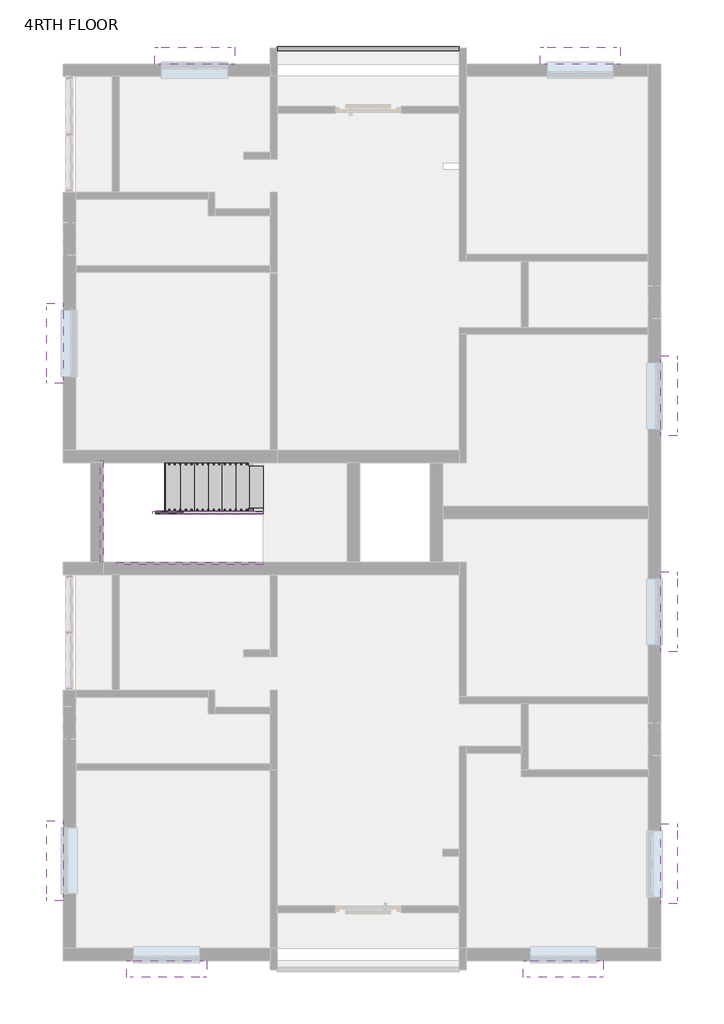
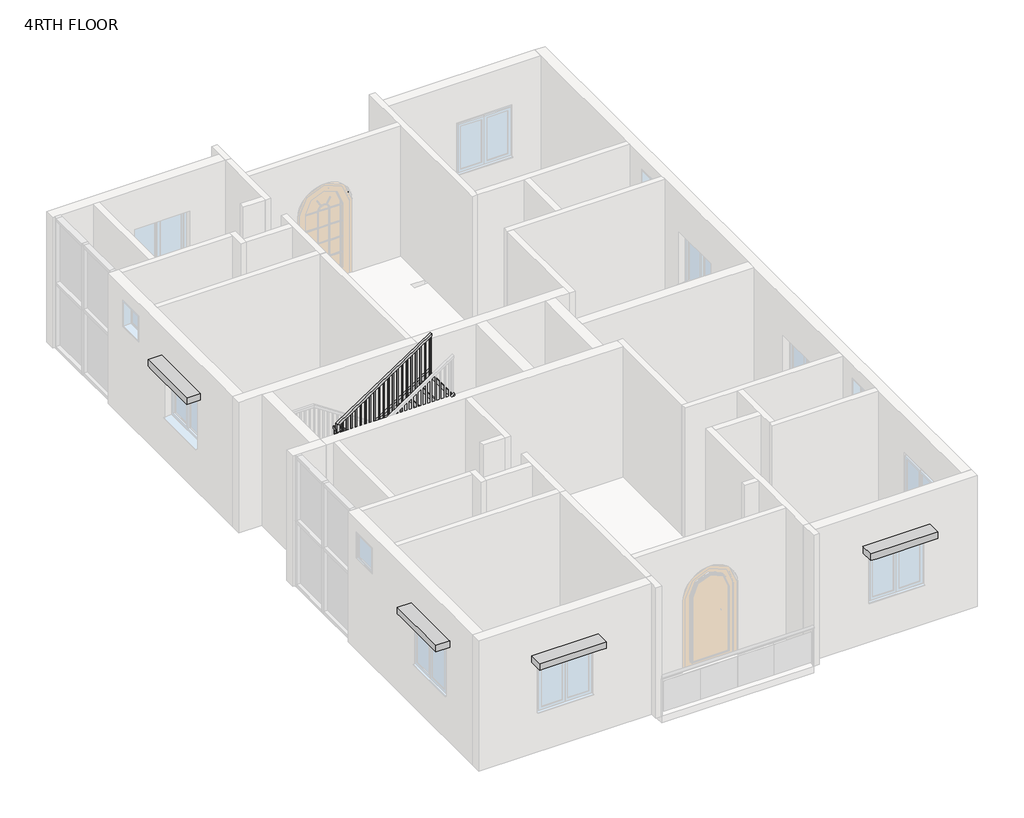
# One storey, part 4 of 4: 9 proxies, 5 members, 2 railings, 1 stair flight.
"""IFC4 building model written with IfcOpenShell, lengths in millimetres."""

from ifc_helpers import new_model, si_unit, point, frame, origin, place, context, project, spatial, polyline, ellipse_curve, trimmed, outline, extrude, faceted_brep, transform, mapped, element, save
from ifc_brep_helpers import plane_surface, extruded_surface, advanced_brep
from components import generic_models_1_generic_models_1_fbb7ad13, generic_models_11_generic_models_11_d301a5e8, generic_models_21_generic_models_21_87948dc1, generic_models_36_generic_models_36_9c63594f, stair_flight_f55dda53

model = new_model("IFC4")

# Units and contexts
model_context = context("Model", 3, world=origin())
ifc_project = project(units=[si_unit("LENGTHUNIT", "METRE", prefix="MILLI")], contexts=[model_context])

# Site, building, storey
site = spatial("IfcSite", under=ifc_project)
building = spatial("IfcBuilding", under=site)
storey = spatial("IfcBuildingStorey", under=building, Name="4RTH FLOOR", Elevation=15240.0)

# Proxies
placement = place(None, origin())
generic_models_1_generic_models_1_shape = generic_models_1_generic_models_1_fbb7ad13(model_context)
element("IfcBuildingElementProxy", 1, Name="Generic Models 1 : Generic Models 1", ObjectType="Generic Models 1 : Generic Models 1", at=placement, inside=storey, context=model_context, shape_type="MappedRepresentation", body=[
    mapped(generic_models_1_generic_models_1_shape, transform((0.0, 0.0, 0.0), x_axis=(1.0, 0.0, 0.0), y_axis=(0.0, 1.0, 0.0), z_axis=(0.0, 0.0, 1.0))),
])
generic_models_11_generic_models_11_shape = generic_models_11_generic_models_11_d301a5e8(model_context)
element("IfcBuildingElementProxy", 2, Name="Generic Models 11 : Generic Models 11", ObjectType="Generic Models 11 : Generic Models 11", at=placement, inside=storey, context=model_context, shape_type="MappedRepresentation", body=[
    mapped(generic_models_11_generic_models_11_shape, transform((0.0, 0.0, 0.0), x_axis=(1.0, 0.0, 0.0), y_axis=(0.0, 1.0, 0.0), z_axis=(0.0, 0.0, 1.0))),
])
element("IfcBuildingElementProxy", 3, Name="Generic Models 12 : Generic Models 11", ObjectType="Generic Models 12 : Generic Models 11", at=placement, inside=storey, context=model_context, shape_type="MappedRepresentation", body=[
    mapped(generic_models_11_generic_models_11_shape, transform((-7101.0359618, 0.0, 0.0), x_axis=(1.0, 0.0, 0.0), y_axis=(0.0, 1.0, 0.0), z_axis=(0.0, 0.0, 1.0))),
])
element("IfcBuildingElementProxy", 4, Name="Generic Models 2 : Generic Models 1", ObjectType="Generic Models 2 : Generic Models 1", at=placement, inside=storey, context=model_context, shape_type="MappedRepresentation", body=[
    mapped(generic_models_1_generic_models_1_shape, transform((7304.0875, 0.0, 0.0), x_axis=(1.0, 0.0, 0.0), y_axis=(0.0, 1.0, 0.0), z_axis=(0.0, 0.0, 1.0))),
])
generic_models_21_generic_models_21_shape = generic_models_21_generic_models_21_87948dc1(model_context)
element("IfcBuildingElementProxy", 5, Name="Generic Models 21 : Generic Models 21", ObjectType="Generic Models 21 : Generic Models 21", at=placement, inside=storey, context=model_context, shape_type="MappedRepresentation", body=[
    mapped(generic_models_21_generic_models_21_shape, transform((0.0, 0.0, 0.0), x_axis=(1.0, 0.0, 0.0), y_axis=(0.0, 1.0, 0.0), z_axis=(0.0, 0.0, 1.0))),
])
element("IfcBuildingElementProxy", 6, Name="Generic Models 22 : Generic Models 21", ObjectType="Generic Models 22 : Generic Models 21", at=placement, inside=storey, context=model_context, shape_type="MappedRepresentation", body=[
    mapped(generic_models_21_generic_models_21_shape, transform((0.0, 4641.85, -85.6), x_axis=(1.0, 0.0, 0.0), y_axis=(0.0, 1.0, 0.0), z_axis=(0.0, 0.0, 1.0))),
])
element("IfcBuildingElementProxy", 7, Name="Generic Models 23 : Generic Models 21", ObjectType="Generic Models 23 : Generic Models 21", at=placement, inside=storey, context=model_context, shape_type="MappedRepresentation", body=[
    mapped(generic_models_21_generic_models_21_shape, transform((0.0, 8616.95, -85.6), x_axis=(1.0, 0.0, 0.0), y_axis=(0.0, 1.0, 0.0), z_axis=(0.0, 0.0, 1.0))),
])
generic_models_36_generic_models_36_shape = generic_models_36_generic_models_36_9c63594f(model_context)
element("IfcBuildingElementProxy", 8, Name="Generic Models 36 : Generic Models 36", ObjectType="Generic Models 36 : Generic Models 36", at=placement, inside=storey, context=model_context, shape_type="MappedRepresentation", body=[
    mapped(generic_models_36_generic_models_36_shape, transform((0.0, 0.0, 0.0), x_axis=(1.0, 0.0, 0.0), y_axis=(0.0, 1.0, 0.0), z_axis=(0.0, 0.0, 1.0))),
])
element("IfcBuildingElementProxy", 9, Name="Generic Models 37 : Generic Models 36", ObjectType="Generic Models 37 : Generic Models 36", at=placement, inside=storey, context=model_context, shape_type="MappedRepresentation", body=[
    mapped(generic_models_36_generic_models_36_shape, transform((0.0, -9525.0, 0.0), x_axis=(1.0, 0.0, 0.0), y_axis=(0.0, 1.0, 0.0), z_axis=(0.0, 0.0, 1.0))),
])

# Members
element("IfcMember", 10, ObjectType="Stringer - 2\" Width", at=placement, inside=storey, context=model_context, shape_type="SweptSolid", body=[
    extrude(outline(polyline([(15240.0, -2748.0012202), (15458.0398409, -2748.0012202), (16778.8398409, -4729.2012202), (16412.5158313, -4729.2012202), (15240.0, -2970.4274732), (15240.0, -2748.0012202)])), frame((0.0, 4990.8309003, 0.0), z_axis=(0.0, 1.0, 0.0), x_axis=(0.0, 0.0, 1.0)), (0.0, 0.0, 1.0), 50.8),
])
element("IfcMember", 11, ObjectType="Stringer - 2\" Width", at=placement, inside=storey, context=model_context, shape_type="SweptSolid", body=[
    extrude(outline(polyline([(16982.0398409, -4780.0012202), (16615.7158313, -4780.0012202), (17970.382498, -2748.0012202), (18336.7065076, -2748.0012202), (16982.0398409, -4780.0012202)])), frame((0.0, 4990.8309003, 0.0), z_axis=(0.0, 1.0, 0.0), x_axis=(0.0, 0.0, 1.0)), (0.0, 0.0, 1.0), 50.8),
])
element("IfcMember", 12, ObjectType="Stringer - 2\" Width", at=placement, inside=storey, context=model_context, shape_type="SweptSolid", body=[
    extrude(outline(polyline([(15240.0, -2748.0012202), (15458.0398409, -2748.0012202), (16840.2, -4821.2414588), (16840.2, -5370.7274732), (15240.0, -2970.4274732), (15240.0, -2748.0012202)])), frame((0.0, 5930.6309003, 0.0), z_axis=(0.0, 1.0, 0.0), x_axis=(0.0, 0.0, 1.0)), (0.0, 0.0, 1.0), 50.8),
])
element("IfcMember", 13, ObjectType="Stringer - 2\" Width", at=placement, inside=storey, context=model_context, shape_type="SweptSolid", body=[
    extrude(outline(polyline([(-5745.2012202, 5981.4309003), (-5694.4012202, 5981.4309003), (-5694.4012202, 4101.8309003), (-5745.2012202, 4101.8309003), (-5745.2012202, 5981.4309003)])), frame((0.0, 0.0, 16535.4), z_axis=(0.0, 0.0, 1.0), x_axis=(1.0, 0.0, 0.0)), (0.0, 0.0, 1.0), 304.8),
])
element("IfcMember", 14, ObjectType="Stringer - 2\" Width", at=placement, inside=storey, context=model_context, shape_type="SweptSolid", body=[
    extrude(outline(polyline([(16535.4, -4900.4749672), (17970.382498, -2748.0012202), (18336.7065076, -2748.0012202), (16535.4, -5449.9609815), (16535.4, -4900.4749672)])), frame((0.0, 4051.0309003, 0.0), z_axis=(0.0, 1.0, 0.0), x_axis=(0.0, 0.0, 1.0)), (0.0, 0.0, 1.0), 50.8),
])

# Railings
element("IfcRailing", 15, ObjectType="Glass Panel - Bottom Fill 2", at=placement, inside=storey, context=model_context, shape_type="SolidModel", body=[
    advanced_brep(
    [(-2494.0012202, 13593.7910566, 16154.4), (-2494.0012202, 13517.5910566, 16154.4), (858.7987798, 13593.7910566, 16154.4), (858.7987798, 13517.5910566, 16154.4)],
    [
        (0, 1, ellipse_curve(frame((-2494.0012202, 13555.6910566, 16154.4), z_axis=(-1.0, 0.0, 0.0), x_axis=(0.0, -1.0, 0.0)), 38.1, 28.575)),
        (1, 0, ellipse_curve(frame((-2494.0012202, 13555.6910566, 16154.4), z_axis=(-1.0, 0.0, 0.0), x_axis=(0.0, -1.0, 0.0)), 38.1, 28.575)),
        (2, 3, ellipse_curve(frame((858.7987798, 13555.6910566, 16154.4), z_axis=(1.0, 0.0, 0.0), x_axis=(0.0, -1.0, 0.0)), 38.1, 28.575)),
        (3, 2, ellipse_curve(frame((858.7987798, 13555.6910566, 16154.4), z_axis=(1.0, 0.0, 0.0), x_axis=(0.0, -1.0, 0.0)), 38.1, 28.575)),
        (0, 2),
        (3, 1),
    ],
    [
        plane_surface(frame((-2494.0012202, 13555.6910566, 16154.4), z_axis=(-1.0, 0.0, 0.0), x_axis=(0.0, 1.0, 0.0))),
        plane_surface(frame((858.7987798, 13555.6910566, 16154.4), z_axis=(1.0, 0.0, 0.0), x_axis=(0.0, 1.0, 0.0))),
        extruded_surface(trimmed(ellipse_curve(frame((858.7987798, 13555.6910566, 16154.4), z_axis=(-1.0, 0.0, 0.0), x_axis=(0.0, -1.0, 0.0)), 38.1, 28.575), [point((858.7987798, 13593.7910566, 16154.4))], [point((858.7987798, 13517.5910566, 16154.4))], True, "CARTESIAN"), (-3352.7999999999997, 0.0, 0.0), 3352.7999999999997),
        extruded_surface(trimmed(ellipse_curve(frame((858.7987798, 13555.6910566, 16154.4), z_axis=(-1.0, 0.0, 0.0), x_axis=(0.0, -1.0, 0.0)), 38.1, 28.575), [point((858.7987798, 13517.5910566, 16154.4))], [point((858.7987798, 13593.7910566, 16154.4))], True, "CARTESIAN"), (-3352.7999999999997, 0.0, 0.0), 3352.7999999999997),
    ],
    [
        (0, [[1, 2]]),
        (1, [[3, 4]]),
        (2, [[-1, 5, -4, 6]]),
        (3, [[-2, -6, -3, -5]]),
    ],
),
    extrude(outline(polyline([(-4.8012202, 13562.2262136), (807.9987798, 13562.2262136), (807.9987798, 13555.8762136), (-4.8012202, 13555.8762136), (-4.8012202, 13562.2262136)])), frame((0.0, 0.0, 15341.6), z_axis=(0.0, 0.0, 1.0), x_axis=(1.0, 0.0, 0.0)), (0.0, 0.0, 1.0), 711.2),
    extrude(outline(polyline([(-817.6012202, 13562.2262136), (-4.8012202, 13562.2262136), (-4.8012202, 13555.8762136), (-817.6012202, 13555.8762136), (-817.6012202, 13562.2262136)])), frame((0.0, 0.0, 15341.6), z_axis=(0.0, 0.0, 1.0), x_axis=(1.0, 0.0, 0.0)), (0.0, 0.0, 1.0), 711.2),
    extrude(outline(polyline([(-1630.4012202, 13562.2262136), (-817.6012202, 13562.2262136), (-817.6012202, 13555.8762136), (-1630.4012202, 13555.8762136), (-1630.4012202, 13562.2262136)])), frame((0.0, 0.0, 15341.6), z_axis=(0.0, 0.0, 1.0), x_axis=(1.0, 0.0, 0.0)), (0.0, 0.0, 1.0), 711.2),
    extrude(outline(polyline([(-2443.2012202, 13562.2262136), (-1630.4012202, 13562.2262136), (-1630.4012202, 13555.8762136), (-2443.2012202, 13555.8762136), (-2443.2012202, 13562.2262136)])), frame((0.0, 0.0, 15341.6), z_axis=(0.0, 0.0, 1.0), x_axis=(1.0, 0.0, 0.0)), (0.0, 0.0, 1.0), 711.2),
    extrude(outline(polyline([(846.0987798, 13546.1660566), (846.0987798, 13565.2160566), (865.1487798, 13565.2160566), (865.1487798, 13546.1660566), (846.0987798, 13546.1660566)])), frame((0.0, 0.0, 15240.0), z_axis=(0.0, 0.0, 1.0), x_axis=(1.0, 0.0, 0.0)), (0.0, 0.0, 1.0), 885.825),
    extrude(outline(polyline([(-2500.3512202, 13546.1660566), (-2500.3512202, 13565.2160566), (-2481.3012202, 13565.2160566), (-2481.3012202, 13546.1660566), (-2500.3512202, 13546.1660566)])), frame((0.0, 0.0, 15240.0), z_axis=(0.0, 0.0, 1.0), x_axis=(1.0, 0.0, 0.0)), (0.0, 0.0, 1.0), 885.825),
])
element("IfcRailing", 16, ObjectType="Handrail - Rectangular", at=placement, inside=storey, context=model_context, shape_type="SolidModel", body=[
    faceted_brep([(-2748.0012202, 5041.6309003, 16323.7333333), (-2748.0012202, 5041.6309003, 16262.6793317), (-2748.0012202, 5092.4309003, 16262.6793317), (-2748.0012202, 5092.4309003, 16323.7333333), (-4703.8012202, 5041.6309003, 17627.6), (-4754.6012202, 5041.6309003, 17600.4126651), (-4754.6012202, 5092.4309003, 17600.4126651), (-4703.8012202, 5092.4309003, 17627.6), (-4703.8012202, 5041.6309003, 17678.4), (-4754.6012202, 5041.6309003, 17627.6), (-4754.6012202, 5092.4309003, 17627.6), (-4703.8012202, 5092.4309003, 17678.4), (-4780.0012202, 5041.6309003, 17678.4), (-4780.0012202, 5041.6309003, 17627.6), (-4830.8012202, 5092.4309003, 17627.6), (-4830.8012202, 5092.4309003, 17678.4), (-4780.0012202, 4990.8309003, 17678.4), (-4830.8012202, 4990.8309003, 17678.4), (-4830.8012202, 4940.0309003, 17627.6), (-4780.0012202, 4940.0309003, 17627.6)], [[[0, 1, 2, 3]], [[1, 0, 4, 5]], [[2, 1, 5, 6]], [[3, 2, 6, 7]], [[0, 3, 7, 4]], [[5, 4, 8, 9]], [[6, 5, 9, 10]], [[7, 6, 10, 11]], [[4, 7, 11, 8]], [[9, 8, 12, 13]], [[10, 9, 13, 14]], [[11, 10, 14, 15]], [[8, 11, 15, 12]], [[16, 17, 18, 19]], [[13, 12, 16, 19]], [[14, 13, 19, 18]], [[15, 14, 18, 17]], [[12, 15, 17, 16]]]),
    faceted_brep([(-4780.0012202, 4990.8309003, 17678.4), (-4780.0012202, 4940.0309003, 17627.6), (-4830.8012202, 4940.0309003, 17627.6), (-4830.8012202, 4990.8309003, 17678.4), (-4780.0012202, 4990.8309003, 17786.6793317), (-4830.8012202, 4990.8309003, 17813.8666667), (-4830.8012202, 4940.0309003, 17813.8666667), (-4780.0012202, 4940.0309003, 17786.6793317)], [[[0, 1, 2, 3]], [[4, 5, 6, 7]], [[1, 0, 4, 7]], [[2, 1, 7, 6]], [[3, 2, 6, 5]], [[0, 3, 5, 4]]]),
    faceted_brep([(-4830.8012202, 4990.8309003, 17813.8666667), (-4780.0012202, 4990.8309003, 17786.6793317), (-4780.0012202, 4940.0309003, 17786.6793317), (-4830.8012202, 4940.0309003, 17813.8666667), (-2748.0012202, 4990.8309003, 19202.4), (-2748.0012202, 4940.0309003, 19202.4), (-2748.0012202, 4940.0309003, 19141.3459984), (-2748.0012202, 4990.8309003, 19141.3459984)], [[[0, 1, 2, 3]], [[4, 5, 6, 7]], [[1, 0, 4, 7]], [[2, 1, 7, 6]], [[3, 2, 6, 5]], [[0, 3, 5, 4]]]),
    extrude(outline(polyline([(19118.0626651, -2782.9262202), (18118.6666667, -2782.9262202), (18118.6666667, -2763.8762202), (19130.7626651, -2763.8762202), (19118.0626651, -2782.9262202)])), frame((0.0, 4955.9059003, 0.0), z_axis=(0.0, 1.0, 0.0), x_axis=(0.0, 0.0, 1.0)), (0.0, 0.0, 1.0), 19.05),
    extrude(outline(polyline([(19050.3293317, -2884.5262202), (18118.6666667, -2884.5262202), (18118.6666667, -2865.4762202), (19063.0293317, -2865.4762202), (19050.3293317, -2884.5262202)])), frame((0.0, 4955.9059003, 0.0), z_axis=(0.0, 1.0, 0.0), x_axis=(0.0, 0.0, 1.0)), (0.0, 0.0, 1.0), 19.05),
    extrude(outline(polyline([(18982.5959984, -2986.1262202), (18118.6666667, -2986.1262202), (18118.6666667, -2967.0762202), (18995.2959984, -2967.0762202), (18982.5959984, -2986.1262202)])), frame((0.0, 4955.9059003, 0.0), z_axis=(0.0, 1.0, 0.0), x_axis=(0.0, 0.0, 1.0)), (0.0, 0.0, 1.0), 19.05),
    extrude(outline(polyline([(18914.8626651, -3087.7262202), (17949.3333333, -3087.7262202), (17949.3333333, -3068.6762202), (18927.5626651, -3068.6762202), (18914.8626651, -3087.7262202)])), frame((0.0, 4955.9059003, 0.0), z_axis=(0.0, 1.0, 0.0), x_axis=(0.0, 0.0, 1.0)), (0.0, 0.0, 1.0), 19.05),
    extrude(outline(polyline([(18847.1293317, -3189.3262202), (17949.3333333, -3189.3262202), (17949.3333333, -3170.2762202), (18859.8293317, -3170.2762202), (18847.1293317, -3189.3262202)])), frame((0.0, 4955.9059003, 0.0), z_axis=(0.0, 1.0, 0.0), x_axis=(0.0, 0.0, 1.0)), (0.0, 0.0, 1.0), 19.05),
    extrude(outline(polyline([(18779.3959984, -3290.9262202), (17780.0, -3290.9262202), (17780.0, -3271.8762202), (18792.0959984, -3271.8762202), (18779.3959984, -3290.9262202)])), frame((0.0, 4955.9059003, 0.0), z_axis=(0.0, 1.0, 0.0), x_axis=(0.0, 0.0, 1.0)), (0.0, 0.0, 1.0), 19.05),
    extrude(outline(polyline([(18711.6626651, -3392.5262202), (17780.0, -3392.5262202), (17780.0, -3373.4762202), (18724.3626651, -3373.4762202), (18711.6626651, -3392.5262202)])), frame((0.0, 4955.9059003, 0.0), z_axis=(0.0, 1.0, 0.0), x_axis=(0.0, 0.0, 1.0)), (0.0, 0.0, 1.0), 19.05),
    extrude(outline(polyline([(18643.9293317, -3494.1262202), (17780.0, -3494.1262202), (17780.0, -3475.0762202), (18656.6293317, -3475.0762202), (18643.9293317, -3494.1262202)])), frame((0.0, 4955.9059003, 0.0), z_axis=(0.0, 1.0, 0.0), x_axis=(0.0, 0.0, 1.0)), (0.0, 0.0, 1.0), 19.05),
    extrude(outline(polyline([(18576.1959984, -3595.7262202), (17610.6666667, -3595.7262202), (17610.6666667, -3576.6762202), (18588.8959984, -3576.6762202), (18576.1959984, -3595.7262202)])), frame((0.0, 4955.9059003, 0.0), z_axis=(0.0, 1.0, 0.0), x_axis=(0.0, 0.0, 1.0)), (0.0, 0.0, 1.0), 19.05),
    extrude(outline(polyline([(18508.4626651, -3697.3262202), (17610.6666667, -3697.3262202), (17610.6666667, -3678.2762202), (18521.1626651, -3678.2762202), (18508.4626651, -3697.3262202)])), frame((0.0, 4955.9059003, 0.0), z_axis=(0.0, 1.0, 0.0), x_axis=(0.0, 0.0, 1.0)), (0.0, 0.0, 1.0), 19.05),
    extrude(outline(polyline([(18440.7293317, -3798.9262202), (17441.3333333, -3798.9262202), (17441.3333333, -3779.8762202), (18453.4293317, -3779.8762202), (18440.7293317, -3798.9262202)])), frame((0.0, 4955.9059003, 0.0), z_axis=(0.0, 1.0, 0.0), x_axis=(0.0, 0.0, 1.0)), (0.0, 0.0, 1.0), 19.05),
    extrude(outline(polyline([(18372.9959984, -3900.5262202), (17441.3333333, -3900.5262202), (17441.3333333, -3881.4762202), (18385.6959984, -3881.4762202), (18372.9959984, -3900.5262202)])), frame((0.0, 4955.9059003, 0.0), z_axis=(0.0, 1.0, 0.0), x_axis=(0.0, 0.0, 1.0)), (0.0, 0.0, 1.0), 19.05),
    extrude(outline(polyline([(18305.2626651, -4002.1262202), (17441.3333333, -4002.1262202), (17441.3333333, -3983.0762202), (18317.9626651, -3983.0762202), (18305.2626651, -4002.1262202)])), frame((0.0, 4955.9059003, 0.0), z_axis=(0.0, 1.0, 0.0), x_axis=(0.0, 0.0, 1.0)), (0.0, 0.0, 1.0), 19.05),
    extrude(outline(polyline([(18237.5293317, -4103.7262202), (17272.0, -4103.7262202), (17272.0, -4084.6762202), (18250.2293317, -4084.6762202), (18237.5293317, -4103.7262202)])), frame((0.0, 4955.9059003, 0.0), z_axis=(0.0, 1.0, 0.0), x_axis=(0.0, 0.0, 1.0)), (0.0, 0.0, 1.0), 19.05),
    extrude(outline(polyline([(18169.7959984, -4205.3262202), (17272.0, -4205.3262202), (17272.0, -4186.2762202), (18182.4959984, -4186.2762202), (18169.7959984, -4205.3262202)])), frame((0.0, 4955.9059003, 0.0), z_axis=(0.0, 1.0, 0.0), x_axis=(0.0, 0.0, 1.0)), (0.0, 0.0, 1.0), 19.05),
    extrude(outline(polyline([(18102.0626651, -4306.9262202), (17102.6666667, -4306.9262202), (17102.6666667, -4287.8762202), (18114.7626651, -4287.8762202), (18102.0626651, -4306.9262202)])), frame((0.0, 4955.9059003, 0.0), z_axis=(0.0, 1.0, 0.0), x_axis=(0.0, 0.0, 1.0)), (0.0, 0.0, 1.0), 19.05),
    extrude(outline(polyline([(18034.3293317, -4408.5262202), (17102.6666667, -4408.5262202), (17102.6666667, -4389.4762202), (18047.0293317, -4389.4762202), (18034.3293317, -4408.5262202)])), frame((0.0, 4955.9059003, 0.0), z_axis=(0.0, 1.0, 0.0), x_axis=(0.0, 0.0, 1.0)), (0.0, 0.0, 1.0), 19.05),
    extrude(outline(polyline([(17966.5959984, -4510.1262202), (17102.6666667, -4510.1262202), (17102.6666667, -4491.0762202), (17979.2959984, -4491.0762202), (17966.5959984, -4510.1262202)])), frame((0.0, 4955.9059003, 0.0), z_axis=(0.0, 1.0, 0.0), x_axis=(0.0, 0.0, 1.0)), (0.0, 0.0, 1.0), 19.05),
    extrude(outline(polyline([(17898.8626651, -4611.7262202), (16933.3333333, -4611.7262202), (16933.3333333, -4592.6762202), (17911.5626651, -4592.6762202), (17898.8626651, -4611.7262202)])), frame((0.0, 4955.9059003, 0.0), z_axis=(0.0, 1.0, 0.0), x_axis=(0.0, 0.0, 1.0)), (0.0, 0.0, 1.0), 19.05),
    extrude(outline(polyline([(17831.1293317, -4713.3262202), (16933.3333333, -4713.3262202), (16933.3333333, -4694.2762202), (17843.8293317, -4694.2762202), (17831.1293317, -4713.3262202)])), frame((0.0, 4955.9059003, 0.0), z_axis=(0.0, 1.0, 0.0), x_axis=(0.0, 0.0, 1.0)), (0.0, 0.0, 1.0), 19.05),
    extrude(outline(polyline([(-4770.4762202, 5057.5059003), (-4789.5262202, 5057.5059003), (-4789.5262202, 5076.5559003), (-4770.4762202, 5076.5559003), (-4770.4762202, 5057.5059003)])), frame((0.0, 0.0, 16764.0), z_axis=(0.0, 0.0, 1.0), x_axis=(1.0, 0.0, 0.0)), (0.0, 0.0, 1.0), 863.6),
    extrude(outline(polyline([(17555.9626651, -4687.9262202), (16594.6666667, -4687.9262202), (16594.6666667, -4668.8762202), (17543.2626651, -4668.8762202), (17555.9626651, -4687.9262202)])), frame((0.0, 5057.5059003, 0.0), z_axis=(0.0, 1.0, 0.0), x_axis=(0.0, 0.0, 1.0)), (0.0, 0.0, 1.0), 19.05),
    extrude(outline(polyline([(17488.2293317, -4586.3262202), (16594.6666667, -4586.3262202), (16594.6666667, -4567.2762202), (17475.5293317, -4567.2762202), (17488.2293317, -4586.3262202)])), frame((0.0, 5057.5059003, 0.0), z_axis=(0.0, 1.0, 0.0), x_axis=(0.0, 0.0, 1.0)), (0.0, 0.0, 1.0), 19.05),
    extrude(outline(polyline([(17420.4959984, -4484.7262202), (16425.3333333, -4484.7262202), (16425.3333333, -4465.6762202), (17407.7959984, -4465.6762202), (17420.4959984, -4484.7262202)])), frame((0.0, 5057.5059003, 0.0), z_axis=(0.0, 1.0, 0.0), x_axis=(0.0, 0.0, 1.0)), (0.0, 0.0, 1.0), 19.05),
    extrude(outline(polyline([(17352.7626651, -4383.1262202), (16425.3333333, -4383.1262202), (16425.3333333, -4364.0762202), (17340.0626651, -4364.0762202), (17352.7626651, -4383.1262202)])), frame((0.0, 5057.5059003, 0.0), z_axis=(0.0, 1.0, 0.0), x_axis=(0.0, 0.0, 1.0)), (0.0, 0.0, 1.0), 19.05),
    extrude(outline(polyline([(17285.0293317, -4281.5262202), (16425.3333333, -4281.5262202), (16425.3333333, -4262.4762202), (17272.3293317, -4262.4762202), (17285.0293317, -4281.5262202)])), frame((0.0, 5057.5059003, 0.0), z_axis=(0.0, 1.0, 0.0), x_axis=(0.0, 0.0, 1.0)), (0.0, 0.0, 1.0), 19.05),
    extrude(outline(polyline([(17217.2959984, -4179.9262202), (16256.0, -4179.9262202), (16256.0, -4160.8762202), (17204.5959984, -4160.8762202), (17217.2959984, -4179.9262202)])), frame((0.0, 5057.5059003, 0.0), z_axis=(0.0, 1.0, 0.0), x_axis=(0.0, 0.0, 1.0)), (0.0, 0.0, 1.0), 19.05),
    extrude(outline(polyline([(17149.5626651, -4078.3262202), (16256.0, -4078.3262202), (16256.0, -4059.2762202), (17136.8626651, -4059.2762202), (17149.5626651, -4078.3262202)])), frame((0.0, 5057.5059003, 0.0), z_axis=(0.0, 1.0, 0.0), x_axis=(0.0, 0.0, 1.0)), (0.0, 0.0, 1.0), 19.05),
    extrude(outline(polyline([(17081.8293317, -3976.7262202), (16086.6666667, -3976.7262202), (16086.6666667, -3957.6762202), (17069.1293317, -3957.6762202), (17081.8293317, -3976.7262202)])), frame((0.0, 5057.5059003, 0.0), z_axis=(0.0, 1.0, 0.0), x_axis=(0.0, 0.0, 1.0)), (0.0, 0.0, 1.0), 19.05),
    extrude(outline(polyline([(17014.0959984, -3875.1262202), (16086.6666667, -3875.1262202), (16086.6666667, -3856.0762202), (17001.3959984, -3856.0762202), (17014.0959984, -3875.1262202)])), frame((0.0, 5057.5059003, 0.0), z_axis=(0.0, 1.0, 0.0), x_axis=(0.0, 0.0, 1.0)), (0.0, 0.0, 1.0), 19.05),
    extrude(outline(polyline([(16946.3626651, -3773.5262202), (16086.6666667, -3773.5262202), (16086.6666667, -3754.4762202), (16933.6626651, -3754.4762202), (16946.3626651, -3773.5262202)])), frame((0.0, 5057.5059003, 0.0), z_axis=(0.0, 1.0, 0.0), x_axis=(0.0, 0.0, 1.0)), (0.0, 0.0, 1.0), 19.05),
    extrude(outline(polyline([(16878.6293317, -3671.9262202), (15917.3333333, -3671.9262202), (15917.3333333, -3652.8762202), (16865.9293317, -3652.8762202), (16878.6293317, -3671.9262202)])), frame((0.0, 5057.5059003, 0.0), z_axis=(0.0, 1.0, 0.0), x_axis=(0.0, 0.0, 1.0)), (0.0, 0.0, 1.0), 19.05),
    extrude(outline(polyline([(16810.8959984, -3570.3262202), (15917.3333333, -3570.3262202), (15917.3333333, -3551.2762202), (16798.1959984, -3551.2762202), (16810.8959984, -3570.3262202)])), frame((0.0, 5057.5059003, 0.0), z_axis=(0.0, 1.0, 0.0), x_axis=(0.0, 0.0, 1.0)), (0.0, 0.0, 1.0), 19.05),
    extrude(outline(polyline([(16743.1626651, -3468.7262202), (15748.0, -3468.7262202), (15748.0, -3449.6762202), (16730.4626651, -3449.6762202), (16743.1626651, -3468.7262202)])), frame((0.0, 5057.5059003, 0.0), z_axis=(0.0, 1.0, 0.0), x_axis=(0.0, 0.0, 1.0)), (0.0, 0.0, 1.0), 19.05),
    extrude(outline(polyline([(16675.4293317, -3367.1262202), (15748.0, -3367.1262202), (15748.0, -3348.0762202), (16662.7293317, -3348.0762202), (16675.4293317, -3367.1262202)])), frame((0.0, 5057.5059003, 0.0), z_axis=(0.0, 1.0, 0.0), x_axis=(0.0, 0.0, 1.0)), (0.0, 0.0, 1.0), 19.05),
    extrude(outline(polyline([(16607.6959984, -3265.5262202), (15748.0, -3265.5262202), (15748.0, -3246.4762202), (16594.9959984, -3246.4762202), (16607.6959984, -3265.5262202)])), frame((0.0, 5057.5059003, 0.0), z_axis=(0.0, 1.0, 0.0), x_axis=(0.0, 0.0, 1.0)), (0.0, 0.0, 1.0), 19.05),
    extrude(outline(polyline([(16539.9626651, -3163.9262202), (15578.6666667, -3163.9262202), (15578.6666667, -3144.8762202), (16527.2626651, -3144.8762202), (16539.9626651, -3163.9262202)])), frame((0.0, 5057.5059003, 0.0), z_axis=(0.0, 1.0, 0.0), x_axis=(0.0, 0.0, 1.0)), (0.0, 0.0, 1.0), 19.05),
    extrude(outline(polyline([(16472.2293317, -3062.3262202), (15578.6666667, -3062.3262202), (15578.6666667, -3043.2762202), (16459.5293317, -3043.2762202), (16472.2293317, -3062.3262202)])), frame((0.0, 5057.5059003, 0.0), z_axis=(0.0, 1.0, 0.0), x_axis=(0.0, 0.0, 1.0)), (0.0, 0.0, 1.0), 19.05),
    extrude(outline(polyline([(16404.4959984, -2960.7262202), (15409.3333333, -2960.7262202), (15409.3333333, -2941.6762202), (16391.7959984, -2941.6762202), (16404.4959984, -2960.7262202)])), frame((0.0, 5057.5059003, 0.0), z_axis=(0.0, 1.0, 0.0), x_axis=(0.0, 0.0, 1.0)), (0.0, 0.0, 1.0), 19.05),
    extrude(outline(polyline([(16336.7626651, -2859.1262202), (15409.3333333, -2859.1262202), (15409.3333333, -2840.0762202), (16324.0626651, -2840.0762202), (16336.7626651, -2859.1262202)])), frame((0.0, 5057.5059003, 0.0), z_axis=(0.0, 1.0, 0.0), x_axis=(0.0, 0.0, 1.0)), (0.0, 0.0, 1.0), 19.05),
    extrude(outline(polyline([(-4795.8762202, 4974.9559003), (-4795.8762202, 4955.9059003), (-4814.9262202, 4955.9059003), (-4814.9262202, 4974.9559003), (-4795.8762202, 4974.9559003)])), frame((0.0, 0.0, 16764.0), z_axis=(0.0, 0.0, 1.0), x_axis=(1.0, 0.0, 0.0)), (0.0, 0.0, 1.0), 863.6),
    extrude(outline(polyline([(-4795.8762202, 5057.5059003), (-4814.9262202, 5057.5059003), (-4814.9262202, 5076.5559003), (-4795.8762202, 5076.5559003), (-4795.8762202, 5057.5059003)])), frame((0.0, 0.0, 16764.0), z_axis=(0.0, 0.0, 1.0), x_axis=(1.0, 0.0, 0.0)), (0.0, 0.0, 1.0), 863.6),
    extrude(outline(polyline([(19128.6459984, -2767.0512202), (18118.6666667, -2767.0512202), (18118.6666667, -2748.0012202), (19141.3459984, -2748.0012202), (19128.6459984, -2767.0512202)])), frame((0.0, 4955.9059003, 0.0), z_axis=(0.0, 1.0, 0.0), x_axis=(0.0, 0.0, 1.0)), (0.0, 0.0, 1.0), 19.05),
    extrude(outline(polyline([(16275.3793317, -2767.0512202), (15409.3333333, -2767.0512202), (15409.3333333, -2748.0012202), (16262.6793317, -2748.0012202), (16275.3793317, -2767.0512202)])), frame((0.0, 5057.5059003, 0.0), z_axis=(0.0, 1.0, 0.0), x_axis=(0.0, 0.0, 1.0)), (0.0, 0.0, 1.0), 19.05),
])

# Stair flight
stair_flight_shape = stair_flight_f55dda53(model_context)
element("IfcStairFlight", 17, ObjectType="2\" Tread 1\" Nosing 1/4\" Riser", at=placement, inside=storey, context=model_context, shape_type="MappedRepresentation", body=[
    mapped(stair_flight_shape, transform((0.0, 0.0, 0.0), x_axis=(1.0, 0.0, 0.0), y_axis=(0.0, 1.0, 0.0), z_axis=(0.0, 0.0, 1.0))),
])

save(model, "model.ifc")

# Revit data of these elements
# Type "Glass Panel - Bottom Fill 2"
#   Assembly Code = "C2010400"
#   built-in parameter 1008612 = 0.0416667 (stored number, unit not read)
#   built-in parameter 1008611 = 0.0416667 (stored number, unit not read)
#   built-in parameter 1008609 = 0.333333 (stored number, unit not read)
#   built-in parameter 1008604 = 0.166667 (stored number, unit not read)
#   built-in parameter 1008603 = 0.166667 (stored number, unit not read)
#   Railing Height = 3' - 0"
#   built-in parameter 1008630 = 2
#   built-in parameter 1008610 = 2
#   built-in parameter 1008618 = Baluster - Square : 3/4"
# Type "Handrail - Rectangular"
#   Assembly Code = "C2010400"
#   built-in parameter 1008612 = 0.0416667 (stored number, unit not read)
#   built-in parameter 1008611 = 0.0416667 (stored number, unit not read)
#   built-in parameter 1008609 = 0.333333 (stored number, unit not read)
#   built-in parameter 1008604 = 0.166667 (stored number, unit not read)
#   built-in parameter 1008603 = 0.166667 (stored number, unit not read)
#   Railing Height = 3' - 0"
#   built-in parameter 1008630 = 2
#   built-in parameter 1008610 = 2
#   built-in parameter 1008618 = Baluster - Square : 3/4"
# Element 1 (IfcBuildingElementProxy, "Generic Models 1 : Generic Models 1")
#   Phase Created = New Construction
#   Materials on its faces: "white"
# Element 2 (IfcBuildingElementProxy, "Generic Models 11 : Generic Models 11")
#   Phase Created = New Construction
#   Materials on its faces: "white"
# Element 3 (IfcBuildingElementProxy, "Generic Models 12 : Generic Models 11")
#   Phase Created = New Construction
#   Materials on its faces: "white"
# Element 4 (IfcBuildingElementProxy, "Generic Models 2 : Generic Models 1")
#   Phase Created = New Construction
#   Materials on its faces: "white"
# Element 5 (IfcBuildingElementProxy, "Generic Models 21 : Generic Models 21")
#   Phase Created = New Construction
#   Materials on its faces: "white"
# Element 6 (IfcBuildingElementProxy, "Generic Models 22 : Generic Models 21")
#   Phase Created = New Construction
#   Materials on its faces: "white"
# Element 7 (IfcBuildingElementProxy, "Generic Models 23 : Generic Models 21")
#   Phase Created = New Construction
#   Materials on its faces: "white"
# Element 8 (IfcBuildingElementProxy, "Generic Models 36 : Generic Models 36")
#   Phase Created = New Construction
#   Materials on its faces: "white"
# Element 9 (IfcBuildingElementProxy, "Generic Models 37 : Generic Models 36")
#   Phase Created = New Construction
#   Materials on its faces: "white"
# Elements 10, 11, 12, 13, 14 (IfcMember, "Stringer - 2\" Width")
#   Phase Created = New Construction
# Element 15 (IfcRailing, "Glass Panel - Bottom Fill 2")
#   Phase Created = New Construction
#   Materials on its faces: "Glass"
# Element 16 (IfcRailing, "Handrail - Rectangular")
#   Phase Created = New Construction
# Element 17 (IfcStairFlight, "2\" Tread 1\" Nosing 1/4\" Riser")
#   Phase Created = New Construction
# Materials
#   "white": class "Generic", colour RGB 120 120 120, transparency 0, Cost = 0
#   "Glass": class "Glass", colour RGB 0 128 192, transparency 0.75, Description = "Soda Lime Glass", Cost = 0
